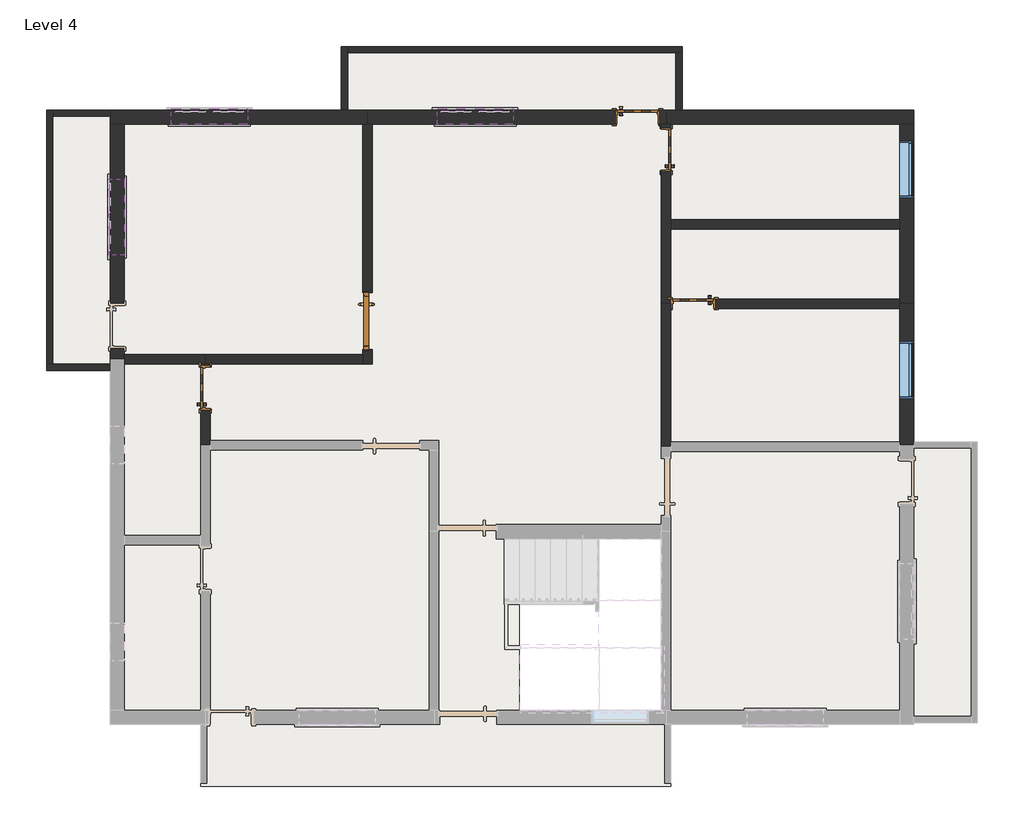
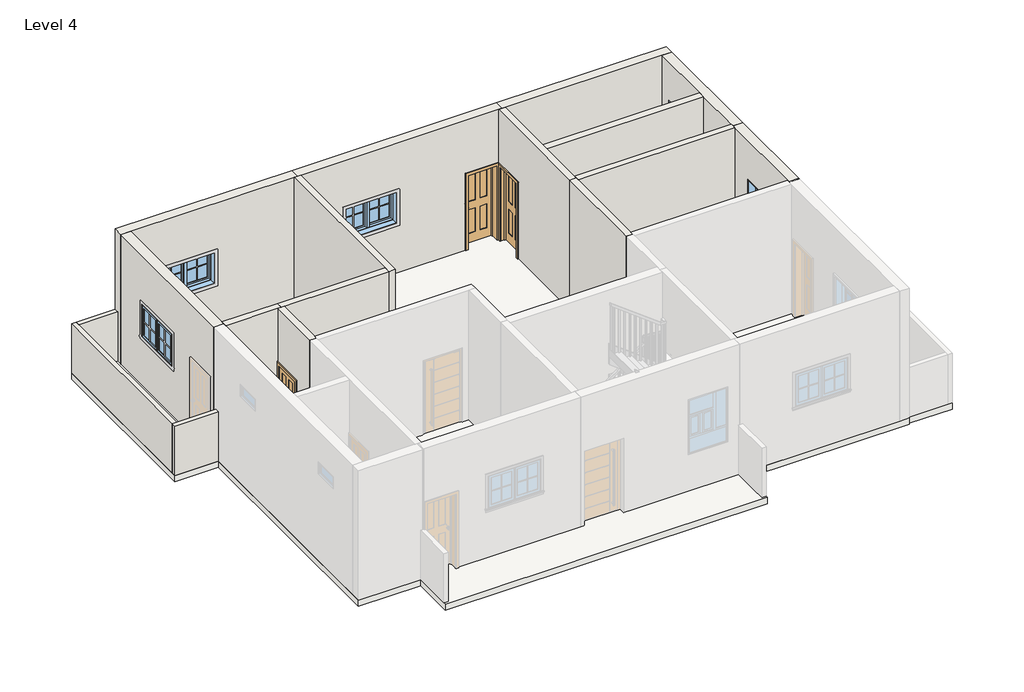
# One storey, part 2 of 3: 20 walls, 5 doors, 5 windows, 1 slab.
"""IFC4 building model written with IfcOpenShell, lengths in millimetres."""

from ifc_helpers import new_model, si_unit, frame, origin, place, context, project, spatial, polyline, outline, extrude, faceted_brep, transform, mapped, element, save
from components import door_3_44036f4b, door_a03dd1d4, door_7109d6db, door_46909e31, m_window_awning_double_horizontal_4_8afcb0b2, m_window_casement_double_sash_variable_3_661e274a

model = new_model("IFC4")

# Units and contexts
model_context = context("Model", 3, world=origin())
ifc_project = project(units=[si_unit("LENGTHUNIT", "METRE", prefix="MILLI")], contexts=[model_context])

# Site, building, storey
site = spatial("IfcSite", under=ifc_project)
building = spatial("IfcBuilding", under=site)
storey = spatial("IfcBuildingStorey", under=building, Name="Level 4", Elevation=9601.2)

# Doors
placement = place(None, origin())
door_3_shape = door_3_44036f4b(model_context)
element("IfcDoor", 1, ObjectType="3'", at=placement, inside=storey, context=model_context, shape_type="MappedRepresentation", body=[
    mapped(door_3_shape, transform((-14176.5794909, 1971.8381491, 9601.2), x_axis=(0.0, -1.0, 0.0), y_axis=(1.0, 0.0, 0.0), z_axis=(0.0, 0.0, 1.0))),
])
door_shape = door_a03dd1d4(model_context)
element("IfcDoor", 2, ObjectType="M_Door-Interior-Single-4_Panel-Wood : 2'2\"", at=placement, inside=storey, context=model_context, shape_type="MappedRepresentation", body=[
    mapped(door_shape, transform((-16770.5544909, 905.4381491, 9601.2), x_axis=(0.0, 1.0, 0.0), y_axis=(-1.0, 0.0, 0.0), z_axis=(0.0, 0.0, 1.0))),
])
door_2_shape = door_7109d6db(model_context)
element("IfcDoor", 3, ObjectType="M_Door-Interior-Single-4_Panel-Wood : 2'2\"", at=placement, inside=storey, context=model_context, shape_type="MappedRepresentation", body=[
    mapped(door_2_shape, transform((-9398.2044909, 4715.4381491, 9601.2), x_axis=(0.0, 1.0, 0.0), y_axis=(-1.0, 0.0, 0.0), z_axis=(0.0, 0.0, 1.0))),
])
element("IfcDoor", 4, ObjectType="M_Door-Interior-Single-4_Panel-Wood : 2'2\"", at=placement, inside=storey, context=model_context, shape_type="MappedRepresentation", body=[
    mapped(door_2_shape, transform((-8969.9794909, 2254.4131491, 9601.2), x_axis=(-1.0, 0.0, 0.0), y_axis=(0.0, -1.0, 0.0), z_axis=(0.0, 0.0, 1.0))),
])
door_4_shape = door_46909e31(model_context)
element("IfcDoor", 5, ObjectType="M_Door-Interior-Single-4_Panel-Wood : 2'2\"", at=placement, inside=storey, context=model_context, shape_type="MappedRepresentation", body=[
    mapped(door_4_shape, transform((-9858.1794909, 5238.9131491, 9601.2), x_axis=(1.0, 0.0, 0.0), y_axis=(0.0, 1.0, 0.0), z_axis=(0.0, 0.0, 1.0))),
])

# Slab
element("IfcSlab", 6, ObjectType="Generic 150mm", at=placement, inside=storey, context=model_context, shape_type="SweptSolid", body=[
    extrude(outline(polyline([(-18291.3794909, 1184.4381491), (-19307.3794909, 1184.4381491), (-19307.3794909, 5350.0381491), (-14596.2721539, 5350.0381491), (-14596.2721539, 6366.0381491), (-9142.3367869, 6366.0381491), (-9142.3367869, 5350.0381491), (-5438.9794909, 5350.0381491), (-5438.9794909, 41.4381491), (-4422.9794909, 41.4381491), (-4422.9794909, -4454.3618509), (-5438.9794909, -4454.3618509), (-5438.9794909, -4479.7618509), (-9325.1794909, -4479.7618509), (-9325.1794909, -5470.3618509), (-16843.5794909, -5470.3618509), (-16843.5794909, -4479.7618509), (-18291.3794909, -4479.7618509), (-18291.3794909, 1184.4381491)]), holes=[polyline([(-11738.1794909, -1507.9618509), (-11738.1794909, -4251.1618509), (-9477.5794909, -4251.1618509), (-9477.5794909, -1507.9618509), (-11738.1794909, -1507.9618509)])]), frame((0.0, 0.0, 9451.2), z_axis=(0.0, 0.0, 1.0), x_axis=(1.0, 0.0, 0.0)), (0.0, 0.0, 1.0), 150.0),
])

# Walls
element("IfcWall", 7, ObjectType="Generic - 4\"", at=placement, inside=storey, context=model_context, shape_type="Brep", body=[
    faceted_brep([(-14494.6721539, 5350.0381491, 9601.2), (-14494.6721539, 6264.4381491, 9601.2), (-14494.6721539, 6366.0381491, 9601.2), (-14494.6721539, 6366.0381491, 10820.4), (-14494.6721539, 6264.4381491, 10820.4), (-14494.6721539, 5350.0381491, 10820.4), (-14596.2721539, 5350.0381491, 9601.2), (-14596.2721539, 5350.0381491, 10820.4), (-14596.2721539, 6366.0381491, 10820.4), (-14596.2721539, 6366.0381491, 9601.2)], [[[0, 1, 2, 3, 4, 5]], [[6, 7, 8, 9]], [[2, 1, 0, 6, 9]], [[5, 4, 3, 8, 7]], [[0, 5, 7, 6]], [[3, 2, 9, 8]]]),
])
element("IfcWall", 8, ObjectType="Generic - 4\"", at=placement, inside=storey, context=model_context, shape_type="Brep", body=[
    faceted_brep([(-14494.6721539, 6264.4381491, 9601.2), (-9243.9367869, 6264.4381491, 9601.2), (-9142.3367869, 6264.4381491, 9601.2), (-9142.3367869, 6264.4381491, 10820.4), (-9243.9367869, 6264.4381491, 10820.4), (-14494.6721539, 6264.4381491, 10820.4), (-14494.6721539, 6366.0381491, 9601.2), (-14494.6721539, 6366.0381491, 10820.4), (-9142.3367869, 6366.0381491, 10820.4), (-9142.3367869, 6366.0381491, 9601.2)], [[[0, 1, 2, 3, 4, 5]], [[6, 7, 8, 9]], [[2, 1, 0, 6, 9]], [[5, 4, 3, 8, 7]], [[0, 5, 7, 6]], [[3, 2, 9, 8]]]),
])
element("IfcWall", 9, ObjectType="Generic - 4\"", at=placement, inside=storey, context=model_context, shape_type="SweptSolid", body=[
    extrude(outline(polyline([(-9243.9367869, 5350.0381491), (-9243.9367869, 6264.4381491), (-9142.3367869, 6264.4381491), (-9142.3367869, 5350.0381491), (-9243.9367869, 5350.0381491)])), frame((0.0, 0.0, 9601.2), z_axis=(0.0, 0.0, 1.0), x_axis=(1.0, 0.0, 0.0)), (0.0, 0.0, 1.0), 1219.2),
])
element("IfcWall", 10, ObjectType="Generic - 4\"", at=placement, inside=storey, context=model_context, shape_type="Brep", body=[
    faceted_brep([(-19307.3794909, 1184.4381491, 9601.2), (-18291.3794909, 1184.4381491, 9601.2), (-18291.3794909, 1184.4381491, 10820.4), (-19307.3794909, 1184.4381491, 10820.4), (-19307.3794909, 1286.0381491, 9601.2), (-19307.3794909, 1286.0381491, 10820.4), (-19205.7794909, 1286.0381491, 10820.4), (-18291.3794909, 1286.0381491, 10820.4), (-18291.3794909, 1286.0381491, 9601.2), (-19205.7794909, 1286.0381491, 9601.2)], [[[0, 1, 2, 3]], [[4, 5, 6, 7, 8, 9]], [[1, 0, 4, 9, 8]], [[3, 2, 7, 6, 5]], [[2, 1, 8, 7]], [[0, 3, 5, 4]]]),
])
element("IfcWall", 11, ObjectType="Generic - 4\"", at=placement, inside=storey, context=model_context, shape_type="Brep", body=[
    faceted_brep([(-19307.3794909, 5350.0381491, 9601.2), (-19307.3794909, 1286.0381491, 9601.2), (-19307.3794909, 1286.0381491, 10820.4), (-19307.3794909, 5350.0381491, 10820.4), (-19205.7794909, 5350.0381491, 9601.2), (-19205.7794909, 5350.0381491, 10820.4), (-19205.7794909, 5248.4381491, 10820.4), (-19205.7794909, 1286.0381491, 10820.4), (-19205.7794909, 1286.0381491, 9601.2), (-19205.7794909, 5248.4381491, 9601.2)], [[[0, 1, 2, 3]], [[4, 5, 6, 7, 8, 9]], [[1, 0, 4, 9, 8]], [[3, 2, 7, 6, 5]], [[2, 1, 8, 7]], [[0, 3, 5, 4]]]),
])
element("IfcWall", 12, ObjectType="Generic - 4\"", at=placement, inside=storey, context=model_context, shape_type="SweptSolid", body=[
    extrude(outline(polyline([(-19205.7794909, 5350.0381491), (-18291.3794909, 5350.0381491), (-18291.3794909, 5248.4381491), (-19205.7794909, 5248.4381491), (-19205.7794909, 5350.0381491)])), frame((0.0, 0.0, 9601.2), z_axis=(0.0, 0.0, 1.0), x_axis=(1.0, 0.0, 0.0)), (0.0, 0.0, 1.0), 1219.2),
])
element("IfcWall", 13, ObjectType="Generic - 6\"", at=placement, inside=storey, context=model_context, shape_type="Brep", body=[
    faceted_brep([(-14252.7794909, 1286.0381491, 12801.6), (-14252.7794909, 1438.4381491, 12801.6), (-14252.7794909, 5121.4381491, 12801.6), (-14252.7794909, 5121.4381491, 9601.2), (-14252.7794909, 2429.0381491, 9601.2), (-14252.7794909, 2429.0381491, 11430.0), (-14252.7794909, 1514.6381491, 11430.0), (-14252.7794909, 1514.6381491, 9601.2), (-14252.7794909, 1438.4381491, 9601.2), (-14252.7794909, 1286.0381491, 9601.2), (-14100.3794909, 5121.4381491, 12801.6), (-14100.3794909, 1286.0381491, 12801.6), (-14100.3794909, 1286.0381491, 9601.2), (-14100.3794909, 1514.6381491, 9601.2), (-14100.3794909, 1514.6381491, 11430.0), (-14100.3794909, 2429.0381491, 11430.0), (-14100.3794909, 2429.0381491, 9601.2), (-14100.3794909, 5121.4381491, 9601.2), (-14232.7794909, 1514.6381491, 9601.2), (-14232.7794909, 1499.6381491, 9601.2), (-14155.7794909, 1499.6381491, 9601.2), (-14155.7794909, 1514.6381491, 9601.2), (-14176.5794909, 5121.4381491, 9601.2), (-14155.7794909, 2429.0381491, 9601.2), (-14155.7794909, 2444.0381491, 9601.2), (-14232.7794909, 2444.0381491, 9601.2), (-14232.7794909, 2429.0381491, 9601.2), (-14176.5794909, 5121.4381491, 12801.6), (-14232.7794909, 2429.0381491, 11430.0), (-14232.7794909, 1514.6381491, 11430.0), (-14155.7794909, 1514.6381491, 11430.0), (-14155.7794909, 2429.0381491, 11430.0), (-14232.7794909, 2444.0381491, 11445.0), (-14155.7794909, 2444.0381491, 11445.0), (-14155.7794909, 1499.6381491, 11445.0), (-14232.7794909, 1499.6381491, 11445.0)], [[[0, 1, 2, 3, 4, 5, 6, 7, 8, 9]], [[10, 11, 12, 13, 14, 15, 16, 17]], [[12, 9, 8, 7, 18, 19, 20, 21, 13]], [[3, 22, 17, 16, 23, 24, 25, 26, 4]], [[2, 1, 0, 11, 10, 27]], [[3, 2, 27, 10, 17, 22]], [[0, 9, 12, 11]], [[5, 28, 29, 6]], [[14, 30, 31, 15]], [[6, 29, 18, 7]], [[30, 14, 13, 21]], [[28, 5, 4, 26]], [[15, 31, 23, 16]], [[32, 33, 34, 35]], [[35, 34, 20, 19]], [[31, 30, 21, 20, 34, 33, 24, 23]], [[33, 32, 25, 24]], [[29, 28, 26, 25, 32, 35, 19, 18]]]),
])
element("IfcWall", 14, ObjectType="Generic - 6\"", at=placement, inside=storey, context=model_context, shape_type="Brep", body=[
    faceted_brep([(-14252.7794909, 1438.4381491, 9601.2), (-16767.3794909, 1438.4381491, 9601.2), (-16767.3794909, 1438.4381491, 12801.6), (-14252.7794909, 1438.4381491, 12801.6), (-14252.7794909, 1286.0381491, 9601.2), (-14252.7794909, 1286.0381491, 12801.6), (-16691.1794909, 1286.0381491, 12801.6), (-16767.3794909, 1286.0381491, 12801.6), (-16767.3794909, 1286.0381491, 9601.2), (-16691.1794909, 1286.0381491, 9601.2)], [[[0, 1, 2, 3]], [[4, 5, 6, 7, 8, 9]], [[1, 0, 4, 9, 8]], [[2, 1, 8, 7]], [[3, 2, 7, 6, 5]], [[0, 3, 5, 4]]]),
])
element("IfcWall", 15, ObjectType="Generic - 6\"", at=placement, inside=storey, context=model_context, shape_type="SweptSolid", body=[
    extrude(outline(polyline([(-5667.5794909, 3445.0381491), (-9325.1794909, 3445.0381491), (-9325.1794909, 3597.4381491), (-5667.5794909, 3597.4381491), (-5667.5794909, 3445.0381491)])), frame((0.0, 0.0, 9601.2), z_axis=(0.0, 0.0, 1.0), x_axis=(1.0, 0.0, 0.0)), (0.0, 0.0, 1.0), 3200.4),
])
element("IfcWall", 16, ObjectType="Generic - 6\"", at=placement, inside=storey, context=model_context, shape_type="Brep", body=[
    faceted_brep([(-9325.1794909, 2327.4381491, 12801.6), (-5667.5794909, 2327.4381491, 12801.6), (-5667.5794909, 2327.4381491, 9601.2), (-8614.7794909, 2327.4381491, 9601.2), (-8614.7794909, 2327.4381491, 11455.0), (-9325.1794909, 2327.4381491, 11455.0), (-5667.5794909, 2175.0381491, 12801.6), (-9325.1794909, 2175.0381491, 12801.6), (-9325.1794909, 2175.0381491, 11455.0), (-8614.7794909, 2175.0381491, 11455.0), (-8614.7794909, 2175.0381491, 9601.2), (-5667.5794909, 2175.0381491, 9601.2), (-5667.5794909, 2251.2381491, 9601.2), (-9325.1794909, 2251.2381491, 12801.6), (-5667.5794909, 2251.2381491, 12801.6)], [[[0, 1, 2, 3, 4, 5]], [[6, 7, 8, 9, 10, 11]], [[2, 12, 11, 10, 3]], [[1, 0, 13, 7, 6, 14]], [[2, 1, 14, 6, 11, 12]], [[7, 13, 0, 5, 8]], [[4, 9, 8, 5]], [[9, 4, 3, 10]]]),
])
element("IfcWall", 17, ObjectType="Generic - 6\"", at=placement, inside=storey, context=model_context, shape_type="Brep", body=[
    faceted_brep([(-9325.1794909, 5121.4381491, 12801.6), (-9325.1794909, 3597.4381491, 12801.6), (-9325.1794909, 3445.0381491, 12801.6), (-9325.1794909, 2327.4381491, 12801.6), (-9325.1794909, 2251.2381491, 12801.6), (-9325.1794909, 2251.2381491, 9601.2), (-9325.1794909, 3445.0381491, 9601.2), (-9325.1794909, 3597.4381491, 9601.2), (-9325.1794909, 4360.2381491, 9601.2), (-9325.1794909, 4360.2381491, 11455.0), (-9325.1794909, 5070.6381491, 11455.0), (-9325.1794909, 5070.6381491, 9601.2), (-9325.1794909, 5121.4381491, 9601.2), (-9477.5794909, 2251.2381491, 12801.6), (-9477.5794909, 5121.4381491, 12801.6), (-9477.5794909, 5121.4381491, 9601.2), (-9477.5794909, 5070.6381491, 9601.2), (-9477.5794909, 5070.6381491, 11455.0), (-9477.5794909, 4360.2381491, 11455.0), (-9477.5794909, 4360.2381491, 9601.2), (-9477.5794909, 2251.2381491, 9601.2), (-9401.3794909, 5121.4381491, 9601.2), (-9401.3794909, 5121.4381491, 12801.6)], [[[0, 1, 2, 3, 4, 5, 6, 7, 8, 9, 10, 11, 12]], [[13, 14, 15, 16, 17, 18, 19, 20]], [[15, 21, 12, 11, 16]], [[5, 20, 19, 8, 7, 6]], [[4, 3, 2, 1, 0, 22, 14, 13]], [[5, 4, 13, 20]], [[0, 12, 21, 15, 14, 22]], [[10, 17, 16, 11]], [[17, 10, 9, 18]], [[18, 9, 8, 19]]]),
])
element("IfcWall", 18, ObjectType="Generic - 6\"", at=placement, inside=storey, context=model_context, shape_type="Brep", body=[
    faceted_brep([(-9325.1794909, -34.7618509, 9601.2), (-9325.1794909, 41.4381491, 9601.2), (-9325.1794909, 2251.2381491, 9601.2), (-9325.1794909, 2251.2381491, 12801.6), (-9325.1794909, 2175.0381491, 12801.6), (-9325.1794909, 41.4381491, 12801.6), (-9325.1794909, -34.7618509, 12801.6), (-9477.5794909, -34.7618509, 9601.2), (-9477.5794909, -34.7618509, 12801.6), (-9477.5794909, 2251.2381491, 12801.6), (-9477.5794909, 2251.2381491, 9601.2)], [[[0, 1, 2, 3, 4, 5, 6]], [[7, 8, 9, 10]], [[2, 1, 0, 7, 10]], [[3, 2, 10, 9]], [[6, 5, 4, 3, 9, 8]], [[0, 6, 8, 7]]]),
])
element("IfcWall", 19, ObjectType="Generic - 6\"", at=placement, inside=storey, context=model_context, shape_type="Brep", body=[
    faceted_brep([(-16691.1794909, 1286.0381491, 12801.6), (-16691.1794909, 66.8381491, 12801.6), (-16691.1794909, -9.3618509, 12801.6), (-16691.1794909, -9.3618509, 9601.2), (-16691.1794909, 66.8381491, 9601.2), (-16691.1794909, 550.2381491, 9601.2), (-16691.1794909, 550.2381491, 11455.0), (-16691.1794909, 1260.6381491, 11455.0), (-16691.1794909, 1260.6381491, 9601.2), (-16691.1794909, 1286.0381491, 9601.2), (-16843.5794909, -9.3618509, 12801.6), (-16843.5794909, 1286.0381491, 12801.6), (-16843.5794909, 1286.0381491, 9601.2), (-16843.5794909, 1260.6381491, 9601.2), (-16843.5794909, 1260.6381491, 11455.0), (-16843.5794909, 550.2381491, 11455.0), (-16843.5794909, 550.2381491, 9601.2), (-16843.5794909, -9.3618509, 9601.2), (-16767.3794909, 1286.0381491, 9601.2), (-16767.3794909, 1286.0381491, 12801.6)], [[[0, 1, 2, 3, 4, 5, 6, 7, 8, 9]], [[10, 11, 12, 13, 14, 15, 16, 17]], [[12, 18, 9, 8, 13]], [[3, 17, 16, 5, 4]], [[2, 1, 0, 19, 11, 10]], [[3, 2, 10, 17]], [[0, 9, 18, 12, 11, 19]], [[7, 14, 13, 8]], [[14, 7, 6, 15]], [[15, 6, 5, 16]]]),
])
element("IfcWall", 20, ObjectType="Generic - 6\"", at=placement, inside=storey, context=model_context, shape_type="Brep", body=[
    faceted_brep([(-16767.3794909, 1438.4381491, 9601.2), (-18062.7794909, 1438.4381491, 9601.2), (-18062.7794909, 1438.4381491, 12801.6), (-16767.3794909, 1438.4381491, 12801.6), (-16767.3794909, 1286.0381491, 9601.2), (-16767.3794909, 1286.0381491, 12801.6), (-16843.5794909, 1286.0381491, 12801.6), (-18062.7794909, 1286.0381491, 12801.6), (-18062.7794909, 1286.0381491, 9601.2), (-16843.5794909, 1286.0381491, 9601.2), (-18062.7794909, 1362.2381491, 9601.2), (-18062.7794909, 1362.2381491, 12801.6)], [[[0, 1, 2, 3]], [[4, 5, 6, 7, 8, 9]], [[1, 0, 4, 9, 8, 10]], [[3, 2, 11, 7, 6, 5]], [[0, 3, 5, 4]], [[2, 1, 10, 8, 7, 11]]]),
])
element("IfcWall", 21, ObjectType="Generic - 9\"", at=placement, inside=storey, context=model_context, shape_type="Brep", body=[
    faceted_brep([(-18291.3794909, 5121.4381491, 12801.6), (-18291.3794909, 5121.4381491, 9601.2), (-18062.7794909, 5121.4381491, 9601.2), (-14252.7794909, 5121.4381491, 9601.2), (-14176.5794909, 5121.4381491, 9601.2), (-14176.5794909, 5121.4381491, 12801.6), (-14252.7794909, 5121.4381491, 12801.6), (-18062.7794909, 5121.4381491, 12801.6), (-16094.2794909, 5121.4381491, 11620.4), (-16094.2794909, 5121.4381491, 10820.4), (-17313.4794909, 5121.4381491, 10820.4), (-17313.4794909, 5121.4381491, 11620.4), (-18291.3794909, 5350.0381491, 9601.2), (-18291.3794909, 5350.0381491, 12801.6), (-14176.5794909, 5350.0381491, 12801.6), (-14176.5794909, 5350.0381491, 9601.2), (-14494.6721539, 5350.0381491, 9601.2), (-14596.2721539, 5350.0381491, 9601.2), (-16094.2794909, 5350.0381491, 11620.4), (-17313.4794909, 5350.0381491, 11620.4), (-17313.4794909, 5350.0381491, 10820.4), (-16094.2794909, 5350.0381491, 10820.4), (-18291.3794909, 5248.4381491, 9601.2)], [[[0, 1, 2, 3, 4, 5, 6, 7], [8, 9, 10, 11]], [[12, 13, 14, 15, 16, 17], [18, 19, 20, 21]], [[4, 3, 2, 1, 22, 12, 17, 16, 15]], [[5, 4, 15, 14]], [[0, 7, 6, 5, 14, 13]], [[0, 13, 12, 22, 1]], [[9, 8, 18, 21]], [[10, 9, 21, 20]], [[11, 10, 20, 19]], [[8, 11, 19, 18]]]),
])
element("IfcWall", 22, ObjectType="Generic - 9\"", at=placement, inside=storey, context=model_context, shape_type="Brep", body=[
    faceted_brep([(-5667.5794909, 5121.4381491, 9601.2), (-5667.5794909, 3597.4381491, 9601.2), (-5667.5794909, 3445.0381491, 9601.2), (-5667.5794909, 2327.4381491, 9601.2), (-5667.5794909, 2251.2381491, 9601.2), (-5667.5794909, 2251.2381491, 12801.6), (-5667.5794909, 2327.4381491, 12801.6), (-5667.5794909, 3445.0381491, 12801.6), (-5667.5794909, 3597.4381491, 12801.6), (-5667.5794909, 5121.4381491, 12801.6), (-5667.5794909, 3943.5131491, 11851.2), (-5667.5794909, 3943.5131491, 10501.2), (-5667.5794909, 4857.9131491, 10501.2), (-5667.5794909, 4857.9131491, 11851.2), (-5438.9794909, 5121.4381491, 9601.2), (-5438.9794909, 5121.4381491, 12801.6), (-5438.9794909, 2251.2381491, 12801.6), (-5438.9794909, 2251.2381491, 9601.2), (-5438.9794909, 3943.5131491, 11851.2), (-5438.9794909, 4857.9131491, 11851.2), (-5438.9794909, 4857.9131491, 10501.2), (-5438.9794909, 3943.5131491, 10501.2)], [[[0, 1, 2, 3, 4, 5, 6, 7, 8, 9], [10, 11, 12, 13]], [[14, 15, 16, 17], [18, 19, 20, 21]], [[4, 3, 2, 1, 0, 14, 17]], [[5, 4, 17, 16]], [[9, 8, 7, 6, 5, 16, 15]], [[0, 9, 15, 14]], [[11, 10, 18, 21]], [[12, 11, 21, 20]], [[13, 12, 20, 19]], [[10, 13, 19, 18]]]),
])
element("IfcWall", 23, ObjectType="Generic - 9\"", at=placement, inside=storey, context=model_context, shape_type="Brep", body=[
    faceted_brep([(-9401.3794909, 5121.4381491, 9601.2), (-9401.3794909, 5121.4381491, 12801.6), (-9477.5794909, 5121.4381491, 12801.6), (-14100.3794909, 5121.4381491, 12801.6), (-14176.5794909, 5121.4381491, 12801.6), (-14176.5794909, 5121.4381491, 9601.2), (-14100.3794909, 5121.4381491, 9601.2), (-10213.3794909, 5121.4381491, 9601.2), (-10213.3794909, 5121.4381491, 11455.0), (-9502.9794909, 5121.4381491, 11455.0), (-9502.9794909, 5121.4381491, 9601.2), (-9477.5794909, 5121.4381491, 9601.2), (-11844.5419909, 5121.4381491, 11620.4), (-11844.5419909, 5121.4381491, 10820.4), (-13063.7419909, 5121.4381491, 10820.4), (-13063.7419909, 5121.4381491, 11620.4), (-9401.3794909, 5350.0381491, 12801.6), (-9401.3794909, 5350.0381491, 9601.2), (-9502.9794909, 5350.0381491, 9601.2), (-9502.9794909, 5350.0381491, 11455.0), (-10213.3794909, 5350.0381491, 11455.0), (-10213.3794909, 5350.0381491, 9601.2), (-14176.5794909, 5350.0381491, 9601.2), (-14176.5794909, 5350.0381491, 12801.6), (-11844.5419909, 5350.0381491, 11620.4), (-13063.7419909, 5350.0381491, 11620.4), (-13063.7419909, 5350.0381491, 10820.4), (-11844.5419909, 5350.0381491, 10820.4)], [[[0, 1, 2, 3, 4, 5, 6, 7, 8, 9, 10, 11], [12, 13, 14, 15]], [[16, 17, 18, 19, 20, 21, 22, 23], [24, 25, 26, 27]], [[5, 22, 21, 7, 6]], [[17, 0, 11, 10, 18]], [[1, 0, 17, 16]], [[4, 3, 2, 1, 16, 23]], [[5, 4, 23, 22]], [[12, 15, 25, 24]], [[15, 14, 26, 25]], [[14, 13, 27, 26]], [[13, 12, 24, 27]], [[9, 19, 18, 10]], [[19, 9, 8, 20]], [[20, 8, 7, 21]]]),
])
element("IfcWall", 24, ObjectType="Generic - 9\"", at=placement, inside=storey, context=model_context, shape_type="Brep", body=[
    faceted_brep([(-9401.3794909, 5121.4381491, 9601.2), (-9325.1794909, 5121.4381491, 9601.2), (-5667.5794909, 5121.4381491, 9601.2), (-5438.9794909, 5121.4381491, 9601.2), (-5438.9794909, 5121.4381491, 12801.6), (-5667.5794909, 5121.4381491, 12801.6), (-9325.1794909, 5121.4381491, 12801.6), (-9401.3794909, 5121.4381491, 12801.6), (-9401.3794909, 5350.0381491, 9601.2), (-9401.3794909, 5350.0381491, 12801.6), (-5438.9794909, 5350.0381491, 12801.6), (-5438.9794909, 5350.0381491, 9601.2), (-9142.3367869, 5350.0381491, 9601.2), (-9243.9367869, 5350.0381491, 9601.2)], [[[0, 1, 2, 3, 4, 5, 6, 7]], [[8, 9, 10, 11, 12, 13]], [[3, 2, 1, 0, 8, 13, 12, 11]], [[7, 6, 5, 4, 10, 9]], [[0, 7, 9, 8]], [[4, 3, 11, 10]]]),
])
element("IfcWall", 25, ObjectType="Generic - 9\"", at=placement, inside=storey, context=model_context, shape_type="Brep", body=[
    faceted_brep([(-5667.5794909, 2251.2381491, 9601.2), (-5667.5794909, 2175.0381491, 9601.2), (-5667.5794909, 41.4381491, 9601.2), (-5667.5794909, -34.7618509, 9601.2), (-5667.5794909, -34.7618509, 12801.6), (-5667.5794909, 41.4381491, 12801.6), (-5667.5794909, 2175.0381491, 12801.6), (-5667.5794909, 2251.2381491, 12801.6), (-5667.5794909, 732.0006491, 11851.2), (-5667.5794909, 732.0006491, 10501.2), (-5667.5794909, 1646.4006491, 10501.2), (-5667.5794909, 1646.4006491, 11851.2), (-5438.9794909, 2251.2381491, 9601.2), (-5438.9794909, 2251.2381491, 12801.6), (-5438.9794909, -34.7618509, 12801.6), (-5438.9794909, -34.7618509, 9601.2), (-5438.9794909, 41.4381491, 9601.2), (-5438.9794909, 732.0006491, 11851.2), (-5438.9794909, 1646.4006491, 11851.2), (-5438.9794909, 1646.4006491, 10501.2), (-5438.9794909, 732.0006491, 10501.2)], [[[0, 1, 2, 3, 4, 5, 6, 7], [8, 9, 10, 11]], [[12, 13, 14, 15, 16], [17, 18, 19, 20]], [[3, 2, 1, 0, 12, 16, 15]], [[7, 6, 5, 4, 14, 13]], [[0, 7, 13, 12]], [[8, 11, 18, 17]], [[11, 10, 19, 18]], [[10, 9, 20, 19]], [[9, 8, 17, 20]], [[3, 15, 14, 4]]]),
])
element("IfcWall", 26, ObjectType="Generic - 9\"", at=placement, inside=storey, context=model_context, shape_type="Brep", body=[
    faceted_brep([(-18062.7794909, 5121.4381491, 12801.6), (-18062.7794909, 1438.4381491, 12801.6), (-18062.7794909, 1362.2381491, 12801.6), (-18062.7794909, 1362.2381491, 9601.2), (-18062.7794909, 1438.4381491, 9601.2), (-18062.7794909, 1540.0381491, 9601.2), (-18062.7794909, 1540.0381491, 11455.0), (-18062.7794909, 2250.4381491, 11455.0), (-18062.7794909, 2250.4381491, 9601.2), (-18062.7794909, 5121.4381491, 9601.2), (-18062.7794909, 4247.5131491, 11620.4), (-18062.7794909, 4247.5131491, 10820.4), (-18062.7794909, 3028.3131491, 10820.4), (-18062.7794909, 3028.3131491, 11620.4), (-18291.3794909, 1362.2381491, 12801.6), (-18291.3794909, 5121.4381491, 12801.6), (-18291.3794909, 5121.4381491, 9601.2), (-18291.3794909, 2250.4381491, 9601.2), (-18291.3794909, 2250.4381491, 11455.0), (-18291.3794909, 1540.0381491, 11455.0), (-18291.3794909, 1540.0381491, 9601.2), (-18291.3794909, 1362.2381491, 9601.2), (-18291.3794909, 4247.5131491, 11620.4), (-18291.3794909, 3028.3131491, 11620.4), (-18291.3794909, 3028.3131491, 10820.4), (-18291.3794909, 4247.5131491, 10820.4)], [[[0, 1, 2, 3, 4, 5, 6, 7, 8, 9], [10, 11, 12, 13]], [[14, 15, 16, 17, 18, 19, 20, 21], [22, 23, 24, 25]], [[16, 9, 8, 17]], [[3, 21, 20, 5, 4]], [[2, 1, 0, 15, 14]], [[9, 16, 15, 0]], [[10, 13, 23, 22]], [[13, 12, 24, 23]], [[12, 11, 25, 24]], [[11, 10, 22, 25]], [[19, 6, 5, 20]], [[6, 19, 18, 7]], [[7, 18, 17, 8]], [[2, 14, 21, 3]]]),
])

# Windows
m_window_awning_double_horizontal_4_shape = m_window_awning_double_horizontal_4_8afcb0b2(model_context)
element("IfcWindow", 27, ObjectType="M_Window-Awning-Double-Horizontal : 4'", at=placement, inside=storey, context=model_context, shape_type="MappedRepresentation", body=[
    mapped(m_window_awning_double_horizontal_4_shape, transform((-16703.8794909, 5235.7381491, 9920.4), x_axis=(1.0, 0.0, 0.0), y_axis=(0.0, 1.0, 0.0), z_axis=(0.0, 0.0, 1.0))),
])
element("IfcWindow", 28, ObjectType="M_Window-Awning-Double-Horizontal : 4'", at=placement, inside=storey, context=model_context, shape_type="MappedRepresentation", body=[
    mapped(m_window_awning_double_horizontal_4_shape, transform((-18177.0794909, 3637.9131491, 9920.4), x_axis=(0.0, 1.0, 0.0), y_axis=(-1.0, 0.0, 0.0), z_axis=(0.0, 0.0, 1.0))),
])
element("IfcWindow", 29, ObjectType="M_Window-Awning-Double-Horizontal : 4'", at=placement, inside=storey, context=model_context, shape_type="MappedRepresentation", body=[
    mapped(m_window_awning_double_horizontal_4_shape, transform((-12454.1419909, 5235.7381491, 9920.4), x_axis=(1.0, 0.0, 0.0), y_axis=(0.0, 1.0, 0.0), z_axis=(0.0, 0.0, 1.0))),
])
m_window_casement_double_sash_variable_3_shape = m_window_casement_double_sash_variable_3_661e274a(model_context)
element("IfcWindow", 30, ObjectType="M_Window-Casement-Double-Sash-Variable : 3'", at=placement, inside=storey, context=model_context, shape_type="MappedRepresentation", body=[
    mapped(m_window_casement_double_sash_variable_3_shape, transform((-5553.2794909, 1189.2006491, 9601.2), x_axis=(0.0, -1.0, 0.0), y_axis=(1.0, 0.0, 0.0), z_axis=(0.0, 0.0, 1.0))),
])
element("IfcWindow", 31, ObjectType="M_Window-Casement-Double-Sash-Variable : 3'", at=placement, inside=storey, context=model_context, shape_type="MappedRepresentation", body=[
    mapped(m_window_casement_double_sash_variable_3_shape, transform((-5553.2794909, 4400.7131491, 9601.2), x_axis=(0.0, -1.0, 0.0), y_axis=(1.0, 0.0, 0.0), z_axis=(0.0, 0.0, 1.0))),
])

save(model, "model.ifc")

# Revit data of these elements
# Type "3'"
#   Type Mark = "41"
#   Water resistance = "up to Class E900, EN 12208:2001"
#   Uniclass2015Version = "v1.21"
#   Uniclass2015Reference = "Ss_25_30_20_30"
#   Uniclass2015Description = "Frame and door leaf system"
#   URL = "www.aluprof.com"
#   Type IFC Predefined Type = "USERDEFINED"
#   Right-hand / Left-hand door [instance default] = ""
#   Resistance to wind load = "up to Class C5/B5, EN 12210:2001"
#   Insert type = "ST"
#   Hardware [instance default] = ""
#   Product page = "https://aluprof.com/en/architects/offer/window-and-door-systems/panel-doors#visualisation"
#   Operation = "SinglePanelOutwardOpening"
#   Opening type = "Outward"
#   NBSReference = "25-50-20/125"
#   NBSDescription = "Frame and door leaf system"
#   Important = "The actual acceptable construction dimensions are dependent on the selection of profiles and hardware, glazing type, construction weight and the construction’s operating conditions. These should be determined by a suitably qualified person, and using ALUPROF’s calculation software"
#   IfcExportType = "USERDEFINED"
#   IfcExportAs = "IfcDoorType"
#   Handle type [instance default] = ""
#   Manufacturer = "ALUPROF SA"
#   Export Type to IFC As = "IfcDoorType"
#   Door sill type [instance default] = ""
#   Description = "External single-leaf panel door outward opening"
#   Model = "MB-86 ST Panel Door AD07"
#   Content of the recyclate in the material = "69.2%"
#   COBie.Type.WarrantyDurationParts = ""
#   COBie.Type.Name = ""
#   COBie.Type.Manufacturer = "ALUPROF SA"
#   COBie.Space.Name = ""
#   COBie.Floor.Name = ""
#   COBie.Facility.Name = ""
#   COBie.CreatedOn = ""
#   COBie.Component.WarrantyStartDate = ""
#   COBie.Component.Name = "MB-86 ST Panel Door AD07"
#   Burglar resistance = "RC2"
#   Air permeability = "up to Class 4, EN 12207:2001"
#   Width of the active leaf = 2' - 8.17717"
#   Placement in wall = 0' - 0.7874"
#   Thickness = 0' - 3.0315"
#   Height of the opening sash = 5' - 9.44094"
#   Handle Offset = 3' - 5.33858"
#   Rough Height = 6' - 2.40945"
#   Rough Width = 3' - 1.1811"
#   Height = 6' - 0"
#   Width = 3' - 0"
#   Construction depth = 0' - 3.0315"
#   Clear opening width = 2' - 3.94882"
#   Clear opening height = 5' - 8.47638"
#   Height of the array = 0' - 11.08136"
#   Schedule No. [instance default] = 1
#   Handrail [instance default] = yes
#   IsExternal = yes
#   Handle [instance default] = no
#   Door closer [instance default] = no
#   Function = 1
#   COBie.Type = yes
#   COBie = yes
#   Access control [instance default] = no
#   Panel = element 361060
#   Wall Closure = (empty or 0)
# Type "M_Door-Interior-Single-4_Panel-Wood : 2'2\""
#   Type Mark = "43"
#   Assembly Code = "C1020300"
#   Analytic Construction = "Wooden"
#   Top Rail = 0' - 4.72441"
#   Thickness = 0' - 1.37795"
#   Thermal Resistance (R) = 0.455703 (m²·K)/W
#   Swing Angle [instance default] = 90.00°
#   Stiles = 0' - 4.72441"
#   Rough Width = 2' - 3.9685"
#   Rough Height = 6' - 0.98425"
#   Mullion = 0' - 4.52756"
#   Lock Rail = 0' - 7.87402"
#   Height = 6' - 0"
#   Width = 2' - 2"
#   Heat Transfer Coefficient (U) = 2.19465 W/(m²·K)
#   Bottom Rail = 0' - 9.05512"
#   Trim Material = Cherry
#   Panel Material = Cherry
#   Frame Material = Cherry
#   Door Handle Material = Aluminum
#   Visual Light Transmittance = 0
#   Solar Heat Gain Coefficient = 0
#   Wall Closure = (empty or 0)
#   Function = (empty or 0)
# Type "Generic 150mm"
#   Function = 0
#   Layers, outside or top first: 0' - 5.90551" no material (function 1)
# Type "Generic - 4\""
#   Layers, outside or top first: 0' - 4" no material (function 1)
# Type "Generic - 6\""
#   Layers, outside or top first: 0' - 6" no material (function 1)
# Type "Generic - 9\""
#   Layers, outside or top first: 0' - 9" no material (function 1)
# Type "M_Window-Awning-Double-Horizontal : 4'"
#   Type Mark = "28"
#   Fire Rating = "0.5h"
#   Assembly Code = "B2020100"
#   Analytic Construction = "Double glazing - domestic"
#   Window Inset [instance default] = 0' - 0"
#   Wall Thickness [instance default] = 0' - 5.90551"
#   Interior Wall Closure [instance default] = 0' - 2.15551"
#   Half Width = 2' - 0"
#   Visual Light Transmittance = 0.81
#   Thermal Resistance (R) = 0.319569 (m²·K)/W
#   Solar Heat Gain Coefficient = 0.76
#   Rough Width = 4' - 0.59055"
#   Rough Height = 2' - 8.08661"
#   Height = 2' - 7.49606"
#   Heat Transfer Coefficient (U) = 3.12929 W/(m²·K)
#   Frame Extension [instance default] = 0' - 0 1/4"
#   Exterior Wall Closure [instance default] = 0' - 1 1/4"
#   Extension Jamb [instance default] = 0' - 2.15551"
#   Default Sill Height = 2' - 11.43307"
#   Width = 4' - 0"
#   Muntin Visibility = yes
#   Interior Trim Visibility [instance default] = yes
#   Exterior Trim Visibility [instance default] = yes
#   Extension Jamb Visibility [instance default] = yes
#   Interior Trim Material = Wood - Stained
#   Muntin Pattern = M_Muntin Pattern_2x2 : M_Muntin Pattern_2x2
#   Interior Trim = M_Trim-Window-Interior-Flat : Picture Frame
#   Interior Frame Material = Wood - Stained
#   Glass Panel Material = Glass
#   Exterior Trim Material = Clad - White
#   Exterior Trim = M_Trim-Window-Exterior-Flat : with Sill
#   Exterior Frame Material = Clad - White
#   Wall Closure = (empty or 0)
# Type "M_Window-Casement-Double-Sash-Variable : 3'"
#   Type Mark = "36"
#   Fire Rating = "0.5h"
#   Assembly Code = "B2020100"
#   Analytic Construction = "Double glazing - domestic"
#   Window Inset [instance default] = 0' - 0 5/8"
#   Wall Thickness [instance default] = 0' - 5.90551"
#   Visual Light Transmittance = 0.81
#   Transom Height Ratio = 0.3
#   Transom Height = 1' - 3.94488"
#   Thermal Resistance (R) = 0.319569 (m²·K)/W
#   Solar Heat Gain Coefficient = 0.76
#   Rough Width = 3' - 0.59055"
#   Rough Height = 4' - 5.74016"
#   Opening Window Height = 1' - 9.25984"
#   Heat Transfer Coefficient (U) = 3.12929 W/(m²·K)
#   Height = 4' - 5.14961"
#   Frame Gap 3 [instance default] = 0' - 1.65041"
#   Frame Gap 2 [instance default] = 0' - 0.62598"
#   Frame Gap 1 = 0' - 1 51/128"
#   Window Width = 1' - 0"
#   Default Sill Height = 2' - 11.43307"
#   Width = 3' - 0"
#   Frame Material = Metal - Aluminum
#   Glass Panel Material = Glass
#   Wall Closure = (empty or 0)
# Element 1 (IfcDoor, "3'")
#   Right-hand / Left-hand door = ""
#   Hardware = ""
#   Handle type = ""
#   Door sill type = ""
#   Schedule No. = 1
#   Handrail = yes
#   Handle = no
#   Door closer = no
#   Access control = no
#   Phase Created = New Construction
# Elements 2, 3, 4, 5 (IfcDoor, "M_Door-Interior-Single-4_Panel-Wood : 2'2\"")
#   Swing Angle = 90.00°
#   Phase Created = New Construction
#   Materials on its faces: "Cherry", "Aluminum"
# Element 6 (IfcSlab, "Generic 150mm")
#   Height Offset From Level = 0' - 0"
#   Phase Created = New Construction
#   Materials on its faces: "WALL2", "Default Floor", "FLOORING TILES 1"
# Elements 7, 8, 9, 10, 12 (IfcWall, "Generic - 4\"")
#   Top Offset = 0' - 0"
#   Base Offset = 0' - 0"
#   Unconnected Height = 4' - 0"
#   wall height = 4' - 0"
#   Phase Created = New Construction
#   Base Constraint = Level 4
#   Materials on its faces: "Default Wall", "WALL2"
# Element 11 (IfcWall, "Generic - 4\"")
#   Top Offset = 0' - 0"
#   Base Offset = 0' - 0"
#   Unconnected Height = 4' - 0"
#   wall height = 4' - 0"
#   Phase Created = New Construction
#   Base Constraint = Level 4
#   Materials on its faces: "WALL2", "Default Wall"
# Element 13 (IfcWall, "Generic - 6\"")
#   Top Offset = 0' - 0"
#   Base Offset = 0' - 0"
#   Unconnected Height = 10' - 6"
#   wall height = 10' - 6"
#   Phase Created = New Construction
#   Base Constraint = Level 4
#   Materials on its faces: "Default Wall", "LIVING 2", "BED ROOM WALL1"
# Element 14 (IfcWall, "Generic - 6\"")
#   Top Offset = 0' - 0"
#   Base Offset = 0' - 0"
#   Unconnected Height = 10' - 6"
#   wall height = 10' - 6"
#   Phase Created = New Construction
#   Base Constraint = Level 4
#   Materials on its faces: "Default Wall", "BED ROOM WALL 2", "LIVING 2"
# Element 15 (IfcWall, "Generic - 6\"")
#   Top Offset = 0' - 0"
#   Base Offset = 0' - 0"
#   Unconnected Height = 10' - 6"
#   wall height = 10' - 6"
#   Phase Created = New Construction
#   Base Constraint = Level 4
#   Materials on its faces: "Default Wall", "BED ROOM WALL 3", "BED ROOM WALL1"
# Elements 16, 17 (IfcWall, "Generic - 6\"")
#   Top Offset = 0' - 0"
#   Base Offset = 0' - 0"
#   Unconnected Height = 10' - 6"
#   wall height = 10' - 6"
#   Phase Created = New Construction
#   Base Constraint = Level 4
#   Materials on its faces: "Default Wall", "BED ROOM WALL1", "LIVING 2"
# Element 18 (IfcWall, "Generic - 6\"")
#   Top Offset = 0' - 0"
#   Base Offset = 0' - 0"
#   Unconnected Height = 10' - 6"
#   wall height = 10' - 6"
#   Phase Created = New Construction
#   Base Constraint = Level 4
#   Materials on its faces: "Default Wall", "LIVING", "LIVING 2"
# Element 19 (IfcWall, "Generic - 6\"")
#   Top Offset = 0' - 0"
#   Base Offset = 0' - 0"
#   Unconnected Height = 10' - 6"
#   wall height = 10' - 6"
#   Phase Created = New Construction
#   Base Constraint = Level 4
#   Materials on its faces: "Default Wall", "LIVING 2", "BATH ROOM WALL 1"
# Element 20 (IfcWall, "Generic - 6\"")
#   Top Offset = 0' - 0"
#   Base Offset = 0' - 0"
#   Unconnected Height = 10' - 6"
#   wall height = 10' - 6"
#   Phase Created = New Construction
#   Base Constraint = Level 4
#   Materials on its faces: "Default Wall", "BED ROOM WALL 2", "BATH ROOM WALL 1"
# Element 21 (IfcWall, "Generic - 9\"")
#   Top Offset = 0' - 0"
#   Base Offset = 0' - 0"
#   Unconnected Height = 10' - 6"
#   wall height = 10' - 6"
#   Phase Created = New Construction
#   Base Constraint = Level 4
#   Materials on its faces: "Default Wall", "WALL2", "BED ROOM WALL1"
# Element 22 (IfcWall, "Generic - 9\"")
#   Top Offset = 0' - 0"
#   Base Offset = 0' - 0"
#   Unconnected Height = 10' - 6"
#   wall height = 10' - 6"
#   Phase Created = New Construction
#   Base Constraint = Level 4
#   Materials on its faces: "Default Wall", "BED ROOM WALL 3", "WALL2"
# Elements 23, 25 (IfcWall, "Generic - 9\"")
#   Top Offset = 0' - 0"
#   Base Offset = 0' - 0"
#   Unconnected Height = 10' - 6"
#   wall height = 10' - 6"
#   Phase Created = New Construction
#   Base Constraint = Level 4
#   Materials on its faces: "Default Wall", "LIVING 2", "WALL2"
# Element 24 (IfcWall, "Generic - 9\"")
#   Top Offset = 0' - 0"
#   Base Offset = 0' - 0"
#   Unconnected Height = 10' - 6"
#   wall height = 10' - 6"
#   Phase Created = New Construction
#   Base Constraint = Level 4
#   Materials on its faces: "Default Wall", "WALL2", "BED ROOM WALL 3"
# Element 26 (IfcWall, "Generic - 9\"")
#   Top Offset = 0' - 0"
#   Base Offset = 0' - 0"
#   Unconnected Height = 10' - 6"
#   wall height = 10' - 6"
#   Phase Created = New Construction
#   Base Constraint = Level 4
#   Materials on its faces: "Default Wall", "BED ROOM WALL 2", "WALL2"
# Element 27 (IfcWindow, "M_Window-Awning-Double-Horizontal : 4'")
#   Mark = "35"
#   Window Inset = 0' - 0"
#   Interior Wall Closure = 0' - 2.15551"
#   Frame Extension = 0' - 0 1/4"
#   Exterior Wall Closure = 0' - 1 1/4"
#   Interior Trim Visibility = yes
#   Exterior Trim Visibility = yes
#   Phase Created = New Construction
#   Materials on its faces: "Wood - Stained", "Glass", "Clad - White"
# Element 28 (IfcWindow, "M_Window-Awning-Double-Horizontal : 4'")
#   Mark = "36"
#   Window Inset = 0' - 0"
#   Interior Wall Closure = 0' - 2.15551"
#   Frame Extension = 0' - 0 1/4"
#   Exterior Wall Closure = 0' - 1 1/4"
#   Interior Trim Visibility = yes
#   Exterior Trim Visibility = yes
#   Phase Created = New Construction
#   Materials on its faces: "Wood - Stained", "Glass", "Clad - White"
# Element 29 (IfcWindow, "M_Window-Awning-Double-Horizontal : 4'")
#   Mark = "37"
#   Window Inset = 0' - 0"
#   Interior Wall Closure = 0' - 2.15551"
#   Frame Extension = 0' - 0 1/4"
#   Exterior Wall Closure = 0' - 1 1/4"
#   Interior Trim Visibility = yes
#   Exterior Trim Visibility = yes
#   Phase Created = New Construction
#   Materials on its faces: "Wood - Stained", "Glass", "Clad - White"
# Element 30 (IfcWindow, "M_Window-Casement-Double-Sash-Variable : 3'")
#   Mark = "41"
#   Window Inset = 0' - 0 5/8"
#   Frame Gap 3 = 0' - 1.65041"
#   Frame Gap 2 = 0' - 0.62598"
#   Phase Created = New Construction
#   Materials on its faces: "Metal - Aluminum", "Glass"
# Element 31 (IfcWindow, "M_Window-Casement-Double-Sash-Variable : 3'")
#   Mark = "42"
#   Window Inset = 0' - 0 5/8"
#   Frame Gap 3 = 0' - 1.65041"
#   Frame Gap 2 = 0' - 0.62598"
#   Phase Created = New Construction
#   Materials on its faces: "Metal - Aluminum", "Glass"
# Materials
#   "Cherry": class "Wood", colour RGB 226 177 128, transparency 0, Description = "Prunus Serotina", Cost = 0
#   "Aluminum": class "Metal", colour RGB 247 247 247, transparency 0, Description = "Aluminum 6061", Cost = 0
#   "Wood - Stained": class "Wood", colour RGB 224 178 126, transparency 0, Cost = 0
#   "Glass": class "Glass", colour RGB 0 128 192, transparency 0.9, Description = "Soda Lime Glass", Cost = 0
#   "Clad - White": class "Wood", colour RGB 242 242 238, transparency 0, Cost = 0
#   "Metal - Aluminum": class "Metal", colour RGB 247 247 247, transparency 0
#   "WALL2": class "Generic", colour RGB 120 120 120, transparency 0, Cost = 0
#   "Default Floor": colour RGB 127 127 127, transparency 0, Cost = 0
#   "FLOORING TILES 1": class "Generic", colour RGB 120 120 120, transparency 0, Cost = 0
#   "Default Wall": colour RGB 128 128 128, transparency 0, Cost = 0
#   "LIVING 2": class "Generic", colour RGB 120 120 120, transparency 0, Cost = 0
#   "BED ROOM WALL1": class "Generic", colour RGB 120 120 120, transparency 0, Cost = 0
#   "BED ROOM WALL 2": class "Generic", colour RGB 120 120 120, transparency 0, Cost = 0
#   "BED ROOM WALL 3": class "Generic", colour RGB 120 120 120, transparency 0, Cost = 0
#   "LIVING": class "Generic", colour RGB 120 120 120, transparency 0, Cost = 0
#   "BATH ROOM WALL 1": class "Generic", colour RGB 120 120 120, transparency 0, Cost = 0
